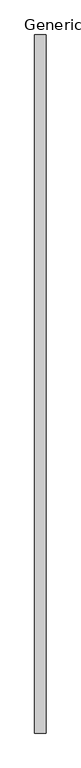
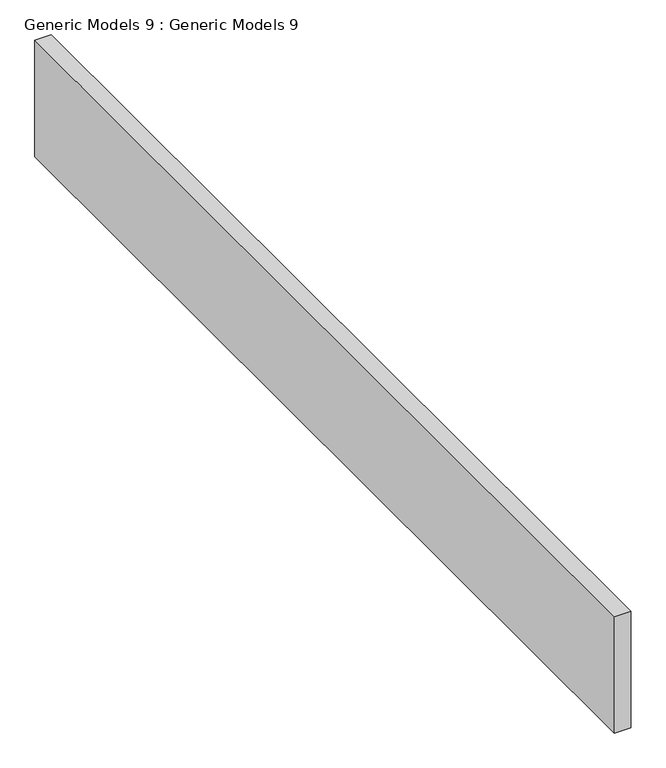
"""IFC4 building model written with IfcOpenShell, lengths in millimetres: proxy geometry, Generic Models 9 : Generic Models 9."""

from ifc_helpers import new_model, si_unit, origin, place, context, project, spatial, faceted_brep, source, transform, mapped, element, save


def generic_models_9_generic_models_9_df2407d9(model_context):
    return source(origin(), model_context, "Body", "Brep", [
        faceted_brep([(-12128.9471301, -9476.6468404, 7057.4337687), (-12215.152412, -9476.6468404, 7057.4337687), (-12215.152412, -14831.2402495, 7057.4337687), (-12128.9471301, -14831.2402495, 7057.4337687), (-12128.9471301, -9476.6468404, 6400.8), (-12128.9471301, -14831.2402495, 6400.8), (-12215.152412, -14831.2402495, 6400.8), (-12215.152412, -9476.6468404, 6400.8), (-12215.152412, -14831.2402495, 7028.6159765)], [[[0, 1, 2, 3]], [[4, 5, 6, 7]], [[1, 0, 4, 7]], [[2, 1, 7, 6, 8]], [[3, 2, 8, 6, 5]], [[0, 3, 5, 4]]]),
    ])


if __name__ == "__main__":
    model = new_model("IFC4")
    model_context = context("Model", 3, world=origin())
    ifc_project = project(units=[si_unit("LENGTHUNIT", "METRE", prefix="MILLI")], contexts=[model_context])
    site = spatial("IfcSite", under=ifc_project)
    building = spatial("IfcBuilding", under=site)
    placement = place(None, origin())
    generic_models_9_generic_models_9_shape = generic_models_9_generic_models_9_df2407d9(model_context)
    element("IfcBuildingElementProxy", 1, Name="Generic Models 9 : Generic Models 9", ObjectType="Generic Models 9 : Generic Models 9", at=placement, inside=building, context=model_context, shape_type="MappedRepresentation", body=[
        mapped(generic_models_9_generic_models_9_shape, transform((0.0, 0.0, 0.0), x_axis=(1.0, 0.0, 0.0), y_axis=(0.0, 1.0, 0.0), z_axis=(0.0, 0.0, 1.0))),
    ])
    save(model, "model.ifc")
